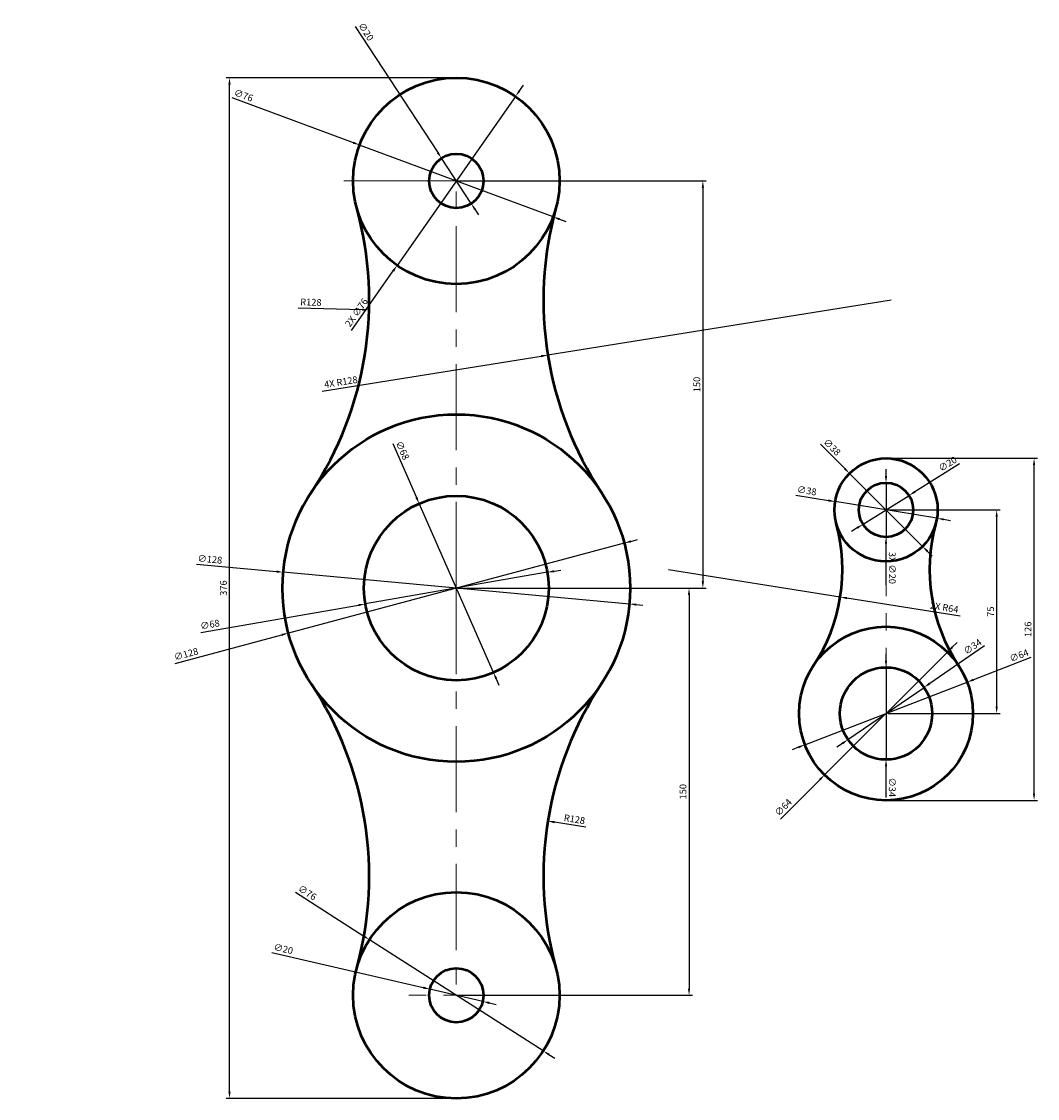
# Model space of a CAD drawing. Units: millimetres. Extents: x 6682 to 7056, y 5969 to 6365.
import ezdxf

# ---------------------------------------------------------------- set-up
doc = ezdxf.new("R2010")
doc.units = ezdxf.units.MM
doc.linetypes.add('CENTER', pattern=[50.8, 31.75, -6.35, 6.35, -6.35])
for name, color, linetype, lineweight in [('M-CNTR', 4, 'CENTER', 18), ('M-DIMS', 2, 'Continuous', 25), ('M-OUTL', 7, 'Continuous', 50)]:
    doc.layers.add(name, color=color, linetype=linetype, lineweight=lineweight)
doc.styles.get("Standard").update_dxf_attribs({"font": 'arial.ttf'})
doc.dimstyles.new('ISO-25', dxfattribs={"dimtxt": 2.5, "dimasz": 2.5, "dimexe": 1.25, "dimexo": 0.625, "dimtad": 1, "dimtxsty": 'Standard', "dimcen": 2.5, "dimadec": 0, "dimazin": 0, "dimtfac": 1, "dimtmove": 0, "dimatfit": 3, "dimfxl": 1, "dimarcsym": 0})

# ---------------------------------------------------------------- blocks, each defined once
blk = doc.blocks.new('*D1')
at = {"layer": 'Defpoints', "color": 0, "transparency": 16777216}
for p in [(7000.25, 6185.6), (7000.25, 6110.6), (7040.98, 6110.6)]:
    blk.add_point(p, dxfattribs=at)
at = {"layer": 'M-DIMS', "color": 0, "lineweight": -2, "transparency": 16777216}
for p, q in [((7000.87, 6185.6), (7042.23, 6185.6)), ((7040.98, 6183.1), (7040.98, 6113.1)), ((7000.87, 6110.6), (7042.23, 6110.6))]:
    blk.add_line(p, q, dxfattribs=at)
at = {"layer": 'M-DIMS', "color": 0, "transparency": 16777216}
for points in [[(7040.57, 6183.1), (7041.4, 6183.1), (7040.98, 6185.6)], [(7040.57, 6113.1), (7041.4, 6113.1), (7040.98, 6110.6)]]:
    blk.add_solid(points, dxfattribs=at)
at = {"layer": 'M-DIMS', "color": 0, "transparency": 16777216, "insert": (7039.09, 6148.1), "char_height": 2.5, "attachment_point": 5, "rotation": 90}
blk.add_mtext('75', dxfattribs=at)
blk = doc.blocks.new('*D2')
at = {"layer": 'Defpoints', "color": 0, "transparency": 16777216}
for p in [(7014.27, 6120.21), (6986.23, 6100.99)]:
    blk.add_point(p, dxfattribs=at)
at = {"layer": 'M-DIMS', "color": 0, "lineweight": -2, "transparency": 16777216}
for p, q in [((7036.51, 6135.47), (7016.33, 6121.63)), ((6986.23, 6100.99), (7014.27, 6120.21)), ((6984.17, 6099.57), (6982.11, 6098.16))]:
    blk.add_line(p, q, dxfattribs=at)
at = {"layer": 'M-DIMS', "color": 0, "transparency": 16777216}
for points in [[(7016.09, 6121.97), (7016.57, 6121.28), (7014.27, 6120.21)], [(6983.93, 6099.91), (6984.4, 6099.23), (6986.23, 6100.99)]]:
    blk.add_solid(points, dxfattribs=at)
at = {"layer": 'M-DIMS', "color": 0, "transparency": 16777216, "insert": (7032.29, 6134.96), "char_height": 2.5, "attachment_point": 5, "rotation": 34.4421}
blk.add_mtext('∅34', dxfattribs=at)
blk = doc.blocks.new('*D3')
at = {"layer": 'Defpoints', "color": 0, "transparency": 16777216}
for p in [(7030.1, 6122.13), (6970.4, 6099.07)]:
    blk.add_point(p, dxfattribs=at)
at = {"layer": 'M-DIMS', "color": 0, "lineweight": -2, "transparency": 16777216}
for p, q in [((7053.56, 6131.18), (7032.43, 6123.03)), ((6970.4, 6099.07), (7030.1, 6122.13)), ((6968.06, 6098.17), (6965.73, 6097.27))]:
    blk.add_line(p, q, dxfattribs=at)
at = {"layer": 'M-DIMS', "color": 0, "transparency": 16777216}
for points in [[(7032.28, 6123.42), (7032.58, 6122.64), (7030.1, 6122.13)], [(6967.91, 6098.56), (6968.21, 6097.78), (6970.4, 6099.07)]]:
    blk.add_solid(points, dxfattribs=at)
at = {"layer": 'M-DIMS', "color": 0, "transparency": 16777216, "insert": (7049.33, 6131.66), "char_height": 2.5, "attachment_point": 5, "rotation": 21.1125}
blk.add_mtext('∅64', dxfattribs=at)
blk = doc.blocks.new('*D4')
at = {"layer": 'Defpoints', "color": 0, "transparency": 16777216}
for p in [(6981.5, 6188.66), (7019, 6182.53)]:
    blk.add_point(p, dxfattribs=at)
at = {"layer": 'M-DIMS', "color": 0, "lineweight": -2, "transparency": 16777216}
for p, q in [((6967, 6191.04), (6979.03, 6189.07)), ((7019, 6182.53), (6981.5, 6188.66)), ((7021.47, 6182.13), (7023.93, 6181.73))]:
    blk.add_line(p, q, dxfattribs=at)
at = {"layer": 'M-DIMS', "color": 0, "transparency": 16777216}
for points in [[(6979.1, 6189.48), (6978.96, 6188.66), (6981.5, 6188.66)], [(7021.53, 6182.54), (7021.4, 6181.72), (7019, 6182.53)]]:
    blk.add_solid(points, dxfattribs=at)
at = {"layer": 'M-DIMS', "color": 0, "transparency": 16777216, "insert": (6971.04, 6192.37), "char_height": 2.5, "attachment_point": 5, "rotation": 350.7162}
blk.add_mtext('∅38', dxfattribs=at)
blk = doc.blocks.new('*D5')
at = {"layer": 'Defpoints', "color": 0, "transparency": 16777216}
for p in [(7008.72, 6190.91), (6991.78, 6180.29)]:
    blk.add_point(p, dxfattribs=at)
at = {"layer": 'M-DIMS', "color": 0, "lineweight": -2, "transparency": 16777216}
for p, q in [((7027.35, 6202.59), (7010.84, 6192.24)), ((6991.78, 6180.29), (7008.72, 6190.91)), ((6989.66, 6178.96), (6987.54, 6177.63))]:
    blk.add_line(p, q, dxfattribs=at)
at = {"layer": 'M-DIMS', "color": 0, "transparency": 16777216}
for points in [[(7010.62, 6192.59), (7011.06, 6191.89), (7008.72, 6190.91)], [(6989.44, 6179.31), (6989.88, 6178.61), (6991.78, 6180.29)]]:
    blk.add_solid(points, dxfattribs=at)
at = {"layer": 'M-DIMS', "color": 0, "transparency": 16777216, "insert": (7023.11, 6202.26), "char_height": 2.5, "attachment_point": 5, "rotation": 32.082}
blk.add_mtext('∅20', dxfattribs=at)
blk = doc.blocks.new('*D6')
at = {"layer": 'Defpoints', "color": 0, "transparency": 16777216}
for p in [(6842.05, 6306.79), (6842.05, 6156.79), (6932.82, 6156.79)]:
    blk.add_point(p, dxfattribs=at)
at = {"layer": 'M-DIMS', "color": 0, "lineweight": -2, "transparency": 16777216}
for p, q in [((6842.67, 6306.79), (6934.07, 6306.79)), ((6932.82, 6304.29), (6932.82, 6159.29)), ((6842.67, 6156.79), (6934.07, 6156.79))]:
    blk.add_line(p, q, dxfattribs=at)
at = {"layer": 'M-DIMS', "color": 0, "transparency": 16777216}
for points in [[(6932.4, 6304.29), (6933.24, 6304.29), (6932.82, 6306.79)], [(6932.4, 6159.29), (6933.24, 6159.29), (6932.82, 6156.79)]]:
    blk.add_solid(points, dxfattribs=at)
at = {"layer": 'M-DIMS', "color": 0, "transparency": 16777216, "insert": (6930.92, 6231.79), "char_height": 2.5, "attachment_point": 5, "rotation": 90}
blk.add_mtext('150', dxfattribs=at)
blk = doc.blocks.new('*D7')
at = {"layer": 'Defpoints', "color": 0, "transparency": 16777216}
for p in [(6806.43, 6320.01), (6877.67, 6293.56)]:
    blk.add_point(p, dxfattribs=at)
at = {"layer": 'M-DIMS', "color": 0, "lineweight": -2, "transparency": 16777216}
for p, q in [((6759.38, 6337.48), (6804.08, 6320.88)), ((6877.67, 6293.56), (6806.43, 6320.01)), ((6880.02, 6292.69), (6882.36, 6291.82))]:
    blk.add_line(p, q, dxfattribs=at)
at = {"layer": 'M-DIMS', "color": 0, "transparency": 16777216}
for points in [[(6804.23, 6321.27), (6803.94, 6320.49), (6806.43, 6320.01)], [(6880.16, 6293.08), (6879.87, 6292.3), (6877.67, 6293.56)]]:
    blk.add_solid(points, dxfattribs=at)
at = {"layer": 'M-DIMS', "color": 0, "transparency": 16777216, "insert": (6763.61, 6338.01), "char_height": 2.5, "attachment_point": 5, "rotation": 339.6328}
blk.add_mtext('∅76', dxfattribs=at)
blk = doc.blocks.new('*D8')
at = {"layer": 'Defpoints', "color": 0, "transparency": 16777216}
for p in [(6836.57, 6315.15), (6847.53, 6298.42)]:
    blk.add_point(p, dxfattribs=at)
at = {"layer": 'M-DIMS', "color": 0, "lineweight": -2, "transparency": 16777216}
for p, q in [((6804.79, 6363.66), (6835.2, 6317.24)), ((6847.53, 6298.42), (6836.57, 6315.15)), ((6848.9, 6296.33), (6850.27, 6294.24))]:
    blk.add_line(p, q, dxfattribs=at)
at = {"layer": 'M-DIMS', "color": 0, "transparency": 16777216}
for points in [[(6835.55, 6317.47), (6834.85, 6317.01), (6836.57, 6315.15)], [(6849.25, 6296.56), (6848.55, 6296.1), (6847.53, 6298.42)]]:
    blk.add_solid(points, dxfattribs=at)
at = {"layer": 'M-DIMS', "color": 0, "transparency": 16777216, "insert": (6808.51, 6361.58), "char_height": 2.5, "attachment_point": 5, "rotation": 303.2296}
blk.add_mtext('∅20', dxfattribs=at)
blk = doc.blocks.new('*D9')
at = {"layer": 'Defpoints', "color": 0, "transparency": 16777216}
for p in [(6875.72, 6070.96), (7002.12, 6050.76)]:
    blk.add_point(p, dxfattribs=at)
at = {"layer": 'M-DIMS', "color": 0, "lineweight": -2, "transparency": 16777216}
blk.add_line((6889.72, 6068.72), (6878.19, 6070.56), dxfattribs=at)
at = {"layer": 'M-DIMS', "color": 0, "transparency": 16777216}
blk.add_solid([(6878.26, 6070.98), (6878.13, 6070.15), (6875.72, 6070.96)], dxfattribs=at)
at = {"layer": 'M-DIMS', "color": 0, "transparency": 16777216, "insert": (6885.49, 6071.32), "char_height": 2.5, "attachment_point": 5, "rotation": 350.9207}
blk.add_mtext('R128', dxfattribs=at)
blk = doc.blocks.new('*D10')
at = {"layer": 'Defpoints', "color": 0, "transparency": 16777216}
for p in [(6842.05, 6156.79), (6842.05, 6006.79), (6927.73, 6006.79)]:
    blk.add_point(p, dxfattribs=at)
at = {"layer": 'M-DIMS', "color": 0, "lineweight": -2, "transparency": 16777216}
for p, q in [((6842.67, 6156.79), (6928.98, 6156.79)), ((6927.73, 6154.29), (6927.73, 6009.29)), ((6842.67, 6006.79), (6928.98, 6006.79))]:
    blk.add_line(p, q, dxfattribs=at)
at = {"layer": 'M-DIMS', "color": 0, "transparency": 16777216}
for points in [[(6927.31, 6154.29), (6928.14, 6154.29), (6927.73, 6156.79)], [(6927.31, 6009.29), (6928.14, 6009.29), (6927.73, 6006.79)]]:
    blk.add_solid(points, dxfattribs=at)
at = {"layer": 'M-DIMS', "color": 0, "transparency": 16777216, "insert": (6925.82, 6081.79), "char_height": 2.5, "attachment_point": 5, "rotation": 90}
blk.add_mtext('150', dxfattribs=at)
blk = doc.blocks.new('*D11')
at = {"layer": 'Defpoints', "color": 0, "transparency": 16777216}
for p in [(6810.04, 6027.27), (6874.06, 5986.3)]:
    blk.add_point(p, dxfattribs=at)
at = {"layer": 'M-DIMS', "color": 0, "lineweight": -2, "transparency": 16777216}
for p, q in [((6782.79, 6044.72), (6807.94, 6028.62)), ((6874.06, 5986.3), (6810.04, 6027.27)), ((6876.16, 5984.95), (6878.27, 5983.61))]:
    blk.add_line(p, q, dxfattribs=at)
at = {"layer": 'M-DIMS', "color": 0, "transparency": 16777216}
for points in [[(6808.16, 6028.97), (6807.71, 6028.27), (6810.04, 6027.27)], [(6876.39, 5985.31), (6875.94, 5984.6), (6874.06, 5986.3)]]:
    blk.add_solid(points, dxfattribs=at)
at = {"layer": 'M-DIMS', "color": 0, "transparency": 16777216, "insert": (6787.03, 6044.34), "char_height": 2.5, "attachment_point": 5, "rotation": 327.3799}
blk.add_mtext('∅76', dxfattribs=at)
blk = doc.blocks.new('*D12')
at = {"layer": 'Defpoints', "color": 0, "transparency": 16777216}
for p in [(6832.31, 6009.05), (6851.79, 6004.53)]:
    blk.add_point(p, dxfattribs=at)
at = {"layer": 'M-DIMS', "color": 0, "lineweight": -2, "transparency": 16777216}
for p, q in [((6774.18, 6022.52), (6829.87, 6009.61)), ((6851.79, 6004.53), (6832.31, 6009.05)), ((6854.23, 6003.96), (6856.66, 6003.4))]:
    blk.add_line(p, q, dxfattribs=at)
at = {"layer": 'M-DIMS', "color": 0, "transparency": 16777216}
for points in [[(6829.97, 6010.02), (6829.78, 6009.2), (6832.31, 6009.05)], [(6854.32, 6004.37), (6854.13, 6003.56), (6851.79, 6004.53)]]:
    blk.add_solid(points, dxfattribs=at)
at = {"layer": 'M-DIMS', "color": 0, "transparency": 16777216, "insert": (6778.3, 6023.59), "char_height": 2.5, "attachment_point": 5, "rotation": 346.9444}
blk.add_mtext('∅20', dxfattribs=at)
blk = doc.blocks.new('*D13')
at = {"layer": 'Defpoints', "color": 0, "transparency": 16777216}
for p in [(6875.55, 6162.6), (6808.55, 6150.98)]:
    blk.add_point(p, dxfattribs=at)
at = {"layer": 'M-DIMS', "color": 0, "lineweight": -2, "transparency": 16777216}
for p, q in [((6875.55, 6162.6), (6808.55, 6150.98)), ((6878.01, 6163.02), (6880.48, 6163.45)), ((6748, 6140.48), (6806.09, 6150.55))]:
    blk.add_line(p, q, dxfattribs=at)
at = {"layer": 'M-DIMS', "color": 0, "transparency": 16777216}
for points in [[(6877.94, 6163.43), (6878.08, 6162.61), (6875.55, 6162.6)], [(6806.01, 6150.96), (6806.16, 6150.14), (6808.55, 6150.98)]]:
    blk.add_solid(points, dxfattribs=at)
at = {"layer": 'M-DIMS', "color": 0, "transparency": 16777216, "insert": (6751.39, 6143.07), "char_height": 2.5, "attachment_point": 5, "rotation": 9.8369}
blk.add_mtext('∅68', dxfattribs=at)
blk = doc.blocks.new('*D14')
at = {"layer": 'Defpoints', "color": 0, "transparency": 16777216}
for p in [(6778.32, 6162.64), (6905.78, 6150.93)]:
    blk.add_point(p, dxfattribs=at)
at = {"layer": 'M-DIMS', "color": 0, "lineweight": -2, "transparency": 16777216}
for p, q in [((6746.4, 6165.57), (6775.83, 6162.87)), ((6905.78, 6150.93), (6778.32, 6162.64)), ((6908.27, 6150.71), (6910.76, 6150.48))]:
    blk.add_line(p, q, dxfattribs=at)
at = {"layer": 'M-DIMS', "color": 0, "transparency": 16777216}
for points in [[(6775.87, 6163.28), (6775.79, 6162.45), (6778.32, 6162.64)], [(6908.31, 6151.12), (6908.23, 6150.29), (6905.78, 6150.93)]]:
    blk.add_solid(points, dxfattribs=at)
at = {"layer": 'M-DIMS', "color": 0, "transparency": 16777216, "insert": (6751.31, 6167.1), "char_height": 2.5, "attachment_point": 5, "rotation": 354.7535}
blk.add_mtext('∅128', dxfattribs=at)
blk = doc.blocks.new('*D15')
at = {"layer": 'Defpoints', "color": 0, "transparency": 16777216}
for p in [(6681.98, 6262.81), (6809.93, 6259.29)]:
    blk.add_point(p, dxfattribs=at)
at = {"layer": 'M-DIMS', "color": 0, "lineweight": -2, "transparency": 16777216}
blk.add_line((6783.87, 6260.01), (6807.43, 6259.36), dxfattribs=at)
at = {"layer": 'M-DIMS', "color": 0, "transparency": 16777216}
blk.add_solid([(6807.44, 6259.78), (6807.42, 6258.95), (6809.93, 6259.29)], dxfattribs=at)
at = {"layer": 'M-DIMS', "color": 0, "transparency": 16777216, "insert": (6788.5, 6261.79), "char_height": 2.5, "attachment_point": 5, "rotation": 358.4245}
blk.add_mtext('R128', dxfattribs=at)
blk = doc.blocks.new('LINK-EYE-76-BORE-20')
for radius in [38, 10]:
    blk.add_circle((38, 38), radius)
blk = doc.blocks.new('*D17')
at = {"layer": 'Defpoints', "color": 0, "transparency": 16777216}
for p in [(6758.54, 6344.79), (6842.05, 6344.79), (6842.05, 5968.79)]:
    blk.add_point(p, dxfattribs=at)
at = {"layer": 'M-DIMS', "color": 0, "lineweight": -2, "transparency": 16777216}
for p, q in [((6841.42, 6344.79), (6757.29, 6344.79)), ((6758.54, 5971.29), (6758.54, 6342.29)), ((6841.42, 5968.79), (6757.29, 5968.79))]:
    blk.add_line(p, q, dxfattribs=at)
at = {"layer": 'M-DIMS', "color": 0, "transparency": 16777216}
for points in [[(6758.12, 6342.29), (6758.96, 6342.29), (6758.54, 6344.79)], [(6758.12, 5971.29), (6758.96, 5971.29), (6758.54, 5968.79)]]:
    blk.add_solid(points, dxfattribs=at)
at = {"layer": 'M-DIMS', "color": 0, "transparency": 16777216, "insert": (6756.64, 6156.79), "char_height": 2.5, "attachment_point": 5, "rotation": 90}
blk.add_mtext('376', dxfattribs=at)
blk = doc.blocks.new('*D18')
at = {"layer": 'Defpoints', "color": 0, "transparency": 16777216}
for p in [(7000.25, 6204.6), (7054.75, 6204.6), (7000.25, 6078.6)]:
    blk.add_point(p, dxfattribs=at)
at = {"layer": 'M-DIMS', "color": 0, "lineweight": -2, "transparency": 16777216}
for p, q in [((7000.87, 6204.6), (7056, 6204.6)), ((7054.75, 6081.1), (7054.75, 6202.1)), ((7000.87, 6078.6), (7056, 6078.6))]:
    blk.add_line(p, q, dxfattribs=at)
at = {"layer": 'M-DIMS', "color": 0, "transparency": 16777216}
for points in [[(7054.33, 6202.1), (7055.17, 6202.1), (7054.75, 6204.6)], [(7054.33, 6081.1), (7055.17, 6081.1), (7054.75, 6078.6)]]:
    blk.add_solid(points, dxfattribs=at)
at = {"layer": 'M-DIMS', "color": 0, "transparency": 16777216, "insert": (7052.85, 6141.6), "char_height": 2.5, "attachment_point": 5, "rotation": 90}
blk.add_mtext('126', dxfattribs=at)
blk = doc.blocks.new('*D19')
at = {"layer": 'Defpoints', "color": 0, "transparency": 16777216}
for p in [(6863.85, 6337.91), (6820.25, 6275.66)]:
    blk.add_point(p, dxfattribs=at)
at = {"layer": 'M-DIMS', "color": 0, "lineweight": -2, "transparency": 16777216}
for p, q in [((6865.28, 6339.96), (6866.72, 6342.01)), ((6863.85, 6337.91), (6820.25, 6275.66)), ((6803.49, 6251.73), (6818.82, 6273.61))]:
    blk.add_line(p, q, dxfattribs=at)
at = {"layer": 'M-DIMS', "color": 0, "transparency": 16777216}
for points in [[(6864.94, 6340.2), (6865.62, 6339.72), (6863.85, 6337.91)], [(6818.48, 6273.85), (6819.16, 6273.37), (6820.25, 6275.66)]]:
    blk.add_solid(points, dxfattribs=at)
at = {"layer": 'M-DIMS', "color": 0, "transparency": 16777216, "insert": (6805.56, 6258.12), "char_height": 2.5, "attachment_point": 5, "rotation": 54.9949}
blk.add_mtext('2X ∅76', dxfattribs=at)
blk = doc.blocks.new('*D20')
at = {"layer": 'Defpoints', "color": 0, "transparency": 16777216}
for p in [(7000.25, 6195.6), (7000.25, 6175.6)]:
    blk.add_point(p, dxfattribs=at)
at = {"layer": 'M-DIMS', "color": 0, "lineweight": -2, "transparency": 16777216}
for p, q in [((7000.25, 6198.1), (7000.25, 6200.6)), ((7000.25, 6195.6), (7000.25, 6175.6)), ((7000.25, 6157.82), (7000.25, 6173.1))]:
    blk.add_line(p, q, dxfattribs=at)
at = {"layer": 'M-DIMS', "color": 0, "transparency": 16777216}
for points in [[(7000.67, 6198.1), (6999.83, 6198.1), (7000.25, 6195.6)], [(7000.67, 6173.1), (6999.83, 6173.1), (7000.25, 6175.6)]]:
    blk.add_solid(points, dxfattribs=at)
at = {"layer": 'M-DIMS', "color": 0, "transparency": 16777216, "insert": (7002.22, 6164.21), "char_height": 2.5, "attachment_point": 5, "rotation": 270.0005}
blk.add_mtext('3X ∅20', dxfattribs=at)
blk = doc.blocks.new('*D21')
at = {"layer": 'Defpoints', "color": 0, "transparency": 16777216}
for p in [(6903.87, 6173.35), (6780.23, 6140.22)]:
    blk.add_point(p, dxfattribs=at)
at = {"layer": 'M-DIMS', "color": 0, "lineweight": -2, "transparency": 16777216}
for p, q in [((6903.87, 6173.35), (6780.23, 6140.22)), ((6906.28, 6174), (6908.7, 6174.65)), ((6738.55, 6129.05), (6777.82, 6139.57))]:
    blk.add_line(p, q, dxfattribs=at)
at = {"layer": 'M-DIMS', "color": 0, "transparency": 16777216}
for points in [[(6906.17, 6174.4), (6906.39, 6173.6), (6903.87, 6173.35)], [(6777.71, 6139.98), (6777.92, 6139.17), (6780.23, 6140.22)]]:
    blk.add_solid(points, dxfattribs=at)
at = {"layer": 'M-DIMS', "color": 0, "transparency": 16777216, "insert": (6742.63, 6132.18), "char_height": 2.5, "attachment_point": 5, "rotation": 15.002}
blk.add_mtext('∅128', dxfattribs=at)
blk = doc.blocks.new('*D22')
at = {"layer": 'Defpoints', "color": 0, "transparency": 16777216}
for p in [(6828.36, 6187.91), (6855.74, 6125.66)]:
    blk.add_point(p, dxfattribs=at)
at = {"layer": 'M-DIMS', "color": 0, "lineweight": -2, "transparency": 16777216}
for p, q in [((6818.63, 6210.04), (6827.35, 6190.2)), ((6855.74, 6125.66), (6828.36, 6187.91)), ((6856.74, 6123.38), (6857.75, 6121.09))]:
    blk.add_line(p, q, dxfattribs=at)
at = {"layer": 'M-DIMS', "color": 0, "transparency": 16777216}
for points in [[(6827.74, 6190.37), (6826.97, 6190.03), (6828.36, 6187.91)], [(6857.13, 6123.54), (6856.36, 6123.21), (6855.74, 6125.66)]]:
    blk.add_solid(points, dxfattribs=at)
at = {"layer": 'M-DIMS', "color": 0, "transparency": 16777216, "insert": (6821.95, 6207.38), "char_height": 2.5, "attachment_point": 5, "rotation": 293.7419}
blk.add_mtext('∅68', dxfattribs=at)
blk = doc.blocks.new('*D23')
at = {"layer": 'Defpoints', "color": 0, "transparency": 16777216}
for p in [(7002.12, 6262.81), (6875.72, 6242.61)]:
    blk.add_point(p, dxfattribs=at)
at = {"layer": 'M-DIMS', "color": 0, "lineweight": -2, "transparency": 16777216}
for p, q in [((7002.12, 6262.81), (6875.72, 6242.61)), ((6792.66, 6229.34), (6873.25, 6242.22))]:
    blk.add_line(p, q, dxfattribs=at)
at = {"layer": 'M-DIMS', "color": 0, "transparency": 16777216}
blk.add_solid([(6873.19, 6242.63), (6873.32, 6241.81), (6875.72, 6242.61)], dxfattribs=at)
at = {"layer": 'M-DIMS', "color": 0, "transparency": 16777216, "insert": (6799.59, 6232.37), "char_height": 2.5, "attachment_point": 5, "rotation": 9.0793}
blk.add_mtext('4X R128', dxfattribs=at)
blk = doc.blocks.new('*D24')
at = {"layer": 'Defpoints', "color": 0, "transparency": 16777216}
for p in [(6986.81, 6199.03), (7013.68, 6172.16)]:
    blk.add_point(p, dxfattribs=at)
at = {"layer": 'M-DIMS', "color": 0, "lineweight": -2, "transparency": 16777216}
for p, q in [((6976.08, 6209.77), (6985.05, 6200.8)), ((7013.68, 6172.16), (6986.81, 6199.03)), ((7015.45, 6170.4), (7017.22, 6168.63))]:
    blk.add_line(p, q, dxfattribs=at)
at = {"layer": 'M-DIMS', "color": 0, "transparency": 16777216}
for points in [[(6985.34, 6201.1), (6984.75, 6200.51), (6986.81, 6199.03)], [(7015.75, 6170.69), (7015.16, 6170.1), (7013.68, 6172.16)]]:
    blk.add_solid(points, dxfattribs=at)
at = {"layer": 'M-DIMS', "color": 0, "transparency": 16777216, "insert": (6980.15, 6208.49), "char_height": 2.5, "attachment_point": 5, "rotation": 314.9994}
blk.add_mtext('∅38', dxfattribs=at)
blk = doc.blocks.new('*D25')
at = {"layer": 'Defpoints', "color": 0, "transparency": 16777216}
for p in [(7022.88, 6133.23), (6977.62, 6087.97)]:
    blk.add_point(p, dxfattribs=at)
at = {"layer": 'M-DIMS', "color": 0, "lineweight": -2, "transparency": 16777216}
for p, q in [((7022.88, 6133.23), (6977.62, 6087.97)), ((7024.64, 6134.99), (7026.41, 6136.76)), ((6961.38, 6071.73), (6975.85, 6086.2))]:
    blk.add_line(p, q, dxfattribs=at)
at = {"layer": 'M-DIMS', "color": 0, "transparency": 16777216}
for points in [[(7024.35, 6135.29), (7024.94, 6134.7), (7022.88, 6133.23)], [(6975.56, 6086.5), (6976.15, 6085.91), (6977.62, 6087.97)]]:
    blk.add_solid(points, dxfattribs=at)
at = {"layer": 'M-DIMS', "color": 0, "transparency": 16777216, "insert": (6962.65, 6075.79), "char_height": 2.5, "attachment_point": 5, "rotation": 44.9999}
blk.add_mtext('∅64', dxfattribs=at)
blk = doc.blocks.new('*D26')
at = {"layer": 'Defpoints', "color": 0, "transparency": 16777216}
for p in [(7000.25, 6127.6), (7000.25, 6093.6)]:
    blk.add_point(p, dxfattribs=at)
at = {"layer": 'M-DIMS', "color": 0, "lineweight": -2, "transparency": 16777216}
for p, q in [((7000.25, 6130.1), (7000.25, 6132.6)), ((7000.25, 6127.6), (7000.25, 6093.6)), ((7000.25, 6079.63), (7000.25, 6091.1))]:
    blk.add_line(p, q, dxfattribs=at)
at = {"layer": 'M-DIMS', "color": 0, "transparency": 16777216}
for points in [[(7000.67, 6130.1), (6999.83, 6130.1), (7000.25, 6127.6)], [(7000.67, 6091.1), (6999.83, 6091.1), (7000.25, 6093.6)]]:
    blk.add_solid(points, dxfattribs=at)
at = {"layer": 'M-DIMS', "color": 0, "transparency": 16777216, "insert": (7002.22, 6083.4), "char_height": 2.5, "attachment_point": 5, "rotation": 270.0003}
blk.add_mtext('∅34', dxfattribs=at)
blk = doc.blocks.new('*D27')
at = {"layer": 'Defpoints', "color": 0, "transparency": 16777216}
for p in [(6920.21, 6163.61), (6983.41, 6153.51)]:
    blk.add_point(p, dxfattribs=at)
at = {"layer": 'M-DIMS', "color": 0, "lineweight": -2, "transparency": 16777216}
for p, q in [((6920.21, 6163.61), (6983.41, 6153.51)), ((7027.57, 6146.46), (6985.88, 6153.12))]:
    blk.add_line(p, q, dxfattribs=at)
at = {"layer": 'M-DIMS', "color": 0, "transparency": 16777216}
blk.add_solid([(6985.95, 6153.53), (6985.82, 6152.71), (6983.41, 6153.51)], dxfattribs=at)
at = {"layer": 'M-DIMS', "color": 0, "transparency": 16777216, "insert": (7021.63, 6149.33), "char_height": 2.5, "attachment_point": 5, "rotation": 350.9208}
blk.add_mtext('2X R64', dxfattribs=at)

msp = doc.modelspace()

# ---------------------------------------------------------------- linework, layer by layer
at = {"layer": 'M-CNTR'}
for p, q in [((6842.049, 6306.787), (6800.686, 6306.787)), ((6800.686, 6306.787), (6886.2, 6306.787)), ((6842.049, 6156.787), (6842.049, 6306.787)), ((7000.249, 6185.6), (7000.249, 6110.6)), ((6842.049, 6156.787), (6842.049, 6006.787)), ((6869.054, 6006.787), (6824.303, 6006.787)), ((6842.049, 6006.787), (6869.054, 6006.787))]:
    msp.add_line(p, q, dxfattribs=at)
at = {"layer": 'M-OUTL'}
for centre, radius in [((6842.049, 6156.787), 64), ((7000.249, 6185.6), 19), ((7000.249, 6185.6), 10), ((6842.049, 6156.787), 34), ((7000.249, 6110.6), 32), ((7000.249, 6110.6), 17)]:
    msp.add_circle(centre, radius, dxfattribs=at)
for centre, radius, start, end in [((6681.98, 6262.813), 128, 326.4804, 15.36099), ((7002.119, 6262.813), 128, 164.63901, 213.5196), ((6920.214, 6163.613), 64, 326.4804, 15.36099), ((7080.284, 6163.613), 64, 164.63901, 213.5196), ((6681.98, 6050.76), 128, 344.63901, 33.5196), ((7002.119, 6050.76), 128, 146.4804, 195.36099)]:
    msp.add_arc(centre, radius, start, end, dxfattribs=at)

# ---------------------------------------------------------------- block references
for p in [(6804.049, 6268.787), (6804.049, 5968.787)]:
    msp.add_blockref('LINK-EYE-76-BORE-20', p, dxfattribs=at)

# ---------------------------------------------------------------- dimensions: what is measured, and where the dimension line sits
at = {"layer": 'M-DIMS'}
for p1, p2, override, picture, middle in [((6847.529, 6298.422), (6836.569, 6315.152), {"dimclrd": 0, "dimclre": 0, "dimclrt": 0}, '*D8', (6806.859, 6360.502)), ((6877.674, 6293.561), (6806.425, 6320.012), {"dimclrd": 0, "dimclre": 0, "dimclrt": 0}, '*D7', (6762.922, 6336.162)), ((6855.738, 6125.664), (6828.36, 6187.909), {"dimdec": 0, "dimlfac": 1, "dimrnd": 0, "dimzin": 0, "dimdsep": 46, "dimlunit": 2}, '*D22', (6820.147, 6206.583)), ((7013.684, 6172.165), (6986.814, 6199.035), {"dimdec": 0, "dimlfac": 1, "dimrnd": 0, "dimzin": 0, "dimdsep": 46, "dimlunit": 2}, '*D24', (6978.753, 6207.096)), ((6991.776, 6180.288), (7008.722, 6190.911), {"dimclrd": 0, "dimclre": 0, "dimclrt": 0}, '*D5', (7024.158, 6200.587)), ((7019, 6182.535), (6981.498, 6188.665), {"dimclrd": 0, "dimclre": 0, "dimclrt": 0}, '*D4', (6970.726, 6190.426)), ((6903.868, 6173.353), (6780.231, 6140.22), {"dimdec": 0, "dimlfac": 1, "dimrnd": 0, "dimzin": 0, "dimdsep": 46, "dimlunit": 2}, '*D21', (6743.139, 6130.28)), ((6905.781, 6150.935), (6778.317, 6162.639), {"dimclrd": 0, "dimclre": 0, "dimclrt": 0}, '*D14', (6751.125, 6165.136)), ((6875.549, 6162.595), (6808.549, 6150.978), {"dimclrd": 0, "dimclre": 0, "dimclrt": 0}, '*D13', (6751.726, 6141.125)), ((6986.229, 6100.985), (7014.269, 6120.215), {"dimclrd": 0, "dimclre": 0, "dimclrt": 0}, '*D2', (7033.402, 6133.336)), ((7022.876, 6133.227), (6977.621, 6087.972), {"dimdec": 0, "dimlfac": 1, "dimrnd": 0, "dimzin": 0, "dimdsep": 46, "dimlunit": 2}, '*D25', (6964.045, 6074.396)), ((6970.397, 6099.073), (7030.101, 6122.126), {"dimclrd": 0, "dimclre": 0, "dimclrt": 0}, '*D3', (7050.042, 6129.826)), ((7000.249, 6127.6), (7000.249, 6093.6), {"dimdec": 0, "dimlfac": 1, "dimrnd": 0, "dimzin": 0, "dimdsep": 46, "dimlunit": 2}, '*D26', (7000.249, 6083.4)), ((6874.055, 5986.302), (6810.043, 6027.271), {"dimclrd": 0, "dimclre": 0, "dimclrt": 0}, '*D11', (6785.965, 6042.682)), ((6851.791, 6004.528), (6832.308, 6009.046), {"dimclrd": 0, "dimclre": 0, "dimclrt": 0}, '*D12', (6777.856, 6021.673))]:
    dim = msp.add_diameter_dim_2p(p1=p1, p2=p2, dimstyle='ISO-25', override=override, dxfattribs=at)
    dim.commit()
    dim.dimension.update_dxf_attribs({"geometry": picture, "text_midpoint": middle, "dimtype": 163})
for base, p1, p2, picture, middle in [((6758.539, 6344.787), (6842.049, 5968.787), (6842.049, 6344.787), '*D17', (6756.636, 6156.787)), ((7054.749, 6204.6), (7000.249, 6078.6), (7000.249, 6204.6), '*D18', (7052.847, 6141.6))]:
    dim = msp.add_linear_dim(base=base, p1=p1, p2=p2, angle=90, dimstyle='ISO-25', override={"dimdec": 0, "dimlfac": 1, "dimrnd": 0, "dimzin": 0, "dimdsep": 46, "dimlunit": 2}, dxfattribs=at)
    dim.commit()
    dim.dimension.update_dxf_attribs({"geometry": picture, "text_midpoint": middle})
dim = msp.add_diameter_dim_2p(p1=(6863.848, 6337.913), p2=(6820.251, 6275.661), text='2X <>', dimstyle='ISO-25', override={"dimdec": 0, "dimlfac": 1, "dimrnd": 0, "dimzin": 0, "dimdsep": 46, "dimlunit": 2}, dxfattribs=at)
dim.commit()
dim.dimension.update_dxf_attribs({"geometry": '*D19', "text_midpoint": (6807.171, 6256.985), "dimtype": 163})
for p1, p2, distance, picture, middle in [((6842.049, 6306.787), (6842.049, 6156.787), 90.771, '*D6', (6930.919, 6231.787)), ((7000.249, 6185.6), (7000.249, 6110.6), 40.733, '*D1', (7039.086, 6148.1)), ((6842.049, 6156.787), (6842.049, 6006.787), 85.677, '*D10', (6925.825, 6081.787))]:
    dim = msp.add_aligned_dim(p1=p1, p2=p2, distance=distance, dimstyle='ISO-25', override={"dimclrd": 0, "dimclre": 0, "dimclrt": 0}, dxfattribs=at)
    dim.commit()
    dim.dimension.update_dxf_attribs({"geometry": picture, "text_midpoint": middle})
for center, mpoint, picture, middle in [((6681.98, 6262.813), (6809.931, 6259.294), '*D15', (6788.453, 6259.885)), ((7002.119, 6050.76), (6875.723, 6070.959), '*D9', (6885.188, 6069.446))]:
    dim = msp.add_radius_dim(center=center, mpoint=mpoint, dimstyle='ISO-25', override={"dimclrd": 0, "dimclre": 0, "dimclrt": 0}, dxfattribs=at)
    dim.commit()
    dim.dimension.update_dxf_attribs({"geometry": picture, "text_midpoint": middle, "dimtype": 164})
for center, mpoint, text, picture, middle in [((7002.119, 6262.813), (6875.723, 6242.615), '4X <>', '*D23', (6799.885, 6230.496)), ((6920.214, 6163.613), (6983.412, 6153.514), '2X <>', '*D27', (7021.331, 6147.454))]:
    dim = msp.add_radius_dim(center=center, mpoint=mpoint, text=text, dimstyle='ISO-25', override={"dimdec": 0, "dimlfac": 1, "dimrnd": 0, "dimzin": 0, "dimdsep": 46, "dimlunit": 2}, dxfattribs=at)
    dim.commit()
    dim.dimension.update_dxf_attribs({"geometry": picture, "text_midpoint": middle, "dimtype": 164})
dim = msp.add_diameter_dim_2p(p1=(7000.249, 6195.6), p2=(7000.249, 6175.6), text='3X <>', dimstyle='ISO-25', override={"dimdec": 0, "dimlfac": 1, "dimrnd": 0, "dimzin": 0, "dimdsep": 46, "dimlunit": 2}, dxfattribs=at)
dim.commit()
dim.dimension.update_dxf_attribs({"geometry": '*D20', "text_midpoint": (7000.249, 6164.21)})

doc.saveas('drawing.dxf')
